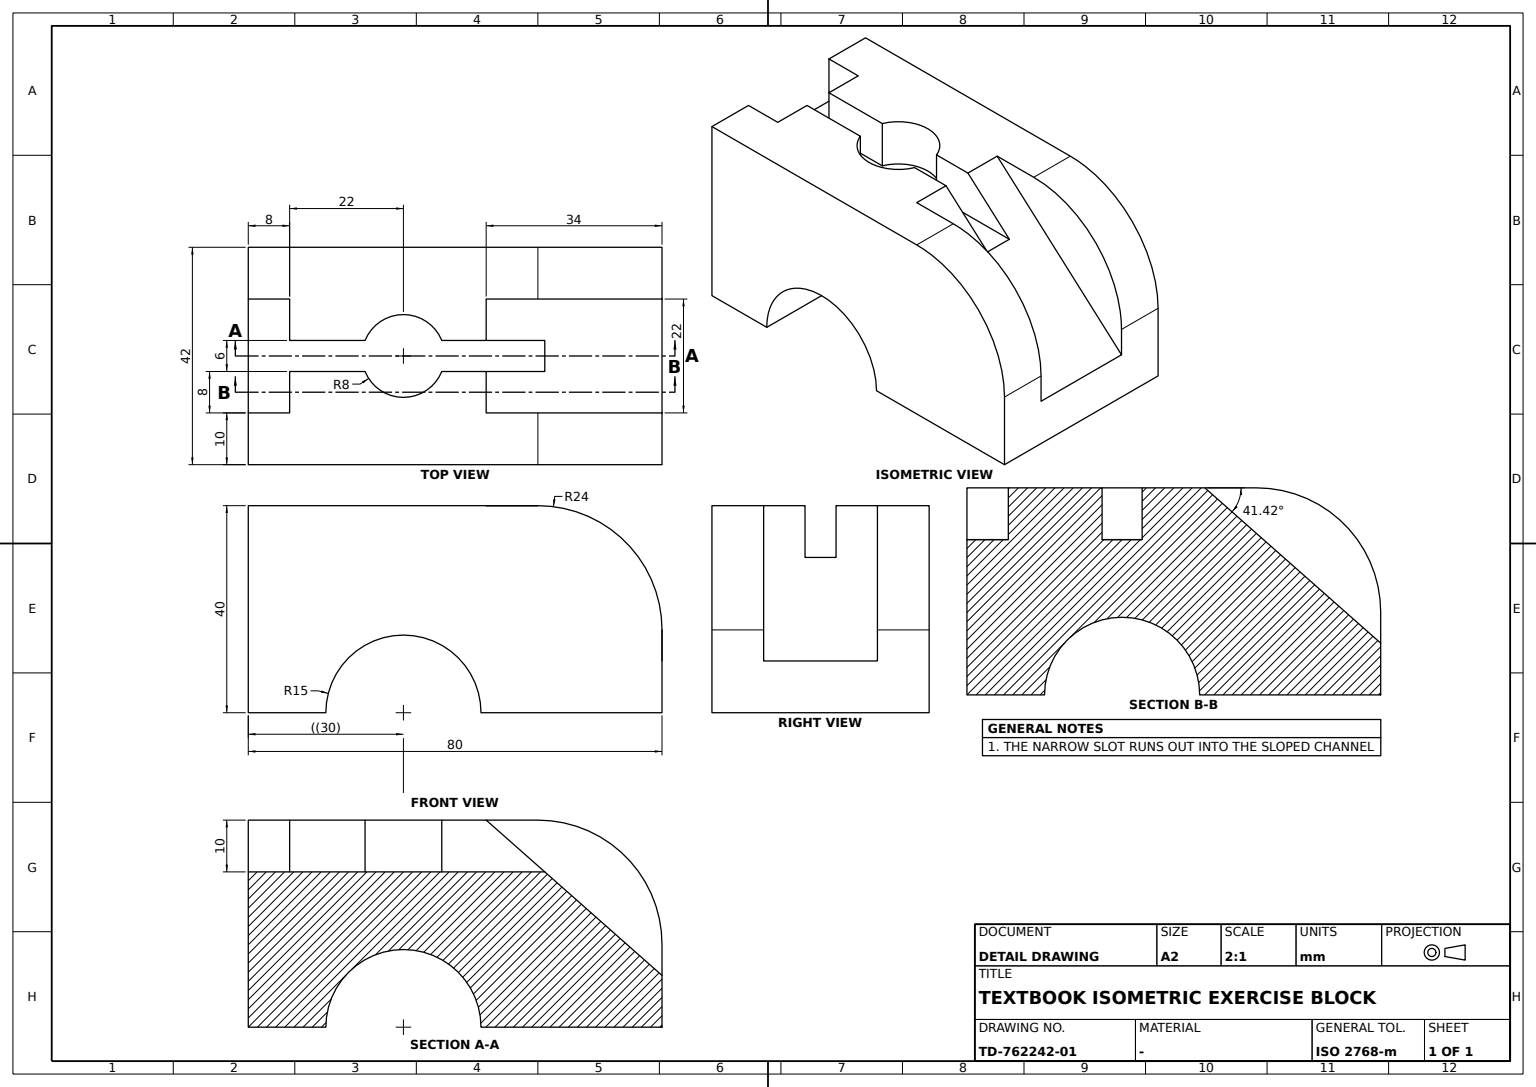
CATIA V5 part; units mm, degrees
sketch "Sketch1" plane through (0, 0, 0) normal (1, 0, 0) x (0, 1, 0)
  line L0 (0, 0) -> (80, 0)
  line L1 (80, 0) -> (80, 40)
  line L2 (80, 40) -> (0, 40)
  line L3 (0, 40) -> (0, 0)
  dimension "length L1" = 40
  dimension "length L0" = 80
  constraint horizontal L0 x-axis
  constraint horizontal L2 x-axis
  constraint vertical L1 y-axis
  constraint vertical L3 y-axis
extrude "Pad1" add sketch "Sketch1" along normal mid plane 42
sketch "Sketch2" plane through (21, 0, 0) normal (1, 0, 0) x (0, 1, 0)
  line L0 (80, 40) -> (46, 40)
  line L1 (46, 40) -> (80, 10)
  line L2 (80, 10) -> (80, 40)
  line L3 (80, 40) -> (0, 40) construction
  line L4 (80, 0) -> (80, 40) construction
  dimension "length L0" = 34
  dimension "length L2" = 30
  constraint horizontal L0 x-axis
  constraint vertical L2 y-axis
  constraint coincidence L0 L3
  constraint coincidence L4 L2
extrude "Pocket1" cut sketch "Sketch2" against normal up to next
sketch "Sketch3" plane through (21, 0, 0) normal (1, 0, 0) x (0, 1, 0)
  line L0 (46, 40) -> (80, 10)
  point P0 (80, 10)
  line L1 (80, 10) -> (80, 40)
  line L2 (80, 40) -> (46, 40)
  line L3 (46, 40) -> (80, 10) construction
  line L4 (80, 0) -> (80, 40) construction
  dimension "length L2" = 34
  constraint vertical L1 y-axis
  constraint horizontal L2 x-axis
  constraint coincidence L0 L3
  constraint coincidence P0 L4
extrude "Pad2" add sketch "Sketch3" against normal blind 10
sketch "Sketch4" plane through (-21, 0, 0) normal (-1, 0, 0) x (0, -1, 0)
  point P0 (-46, 40)
  line L0 (-46, 40) -> (-80, 10)
  line L1 (-80, 10) -> (-80, 40)
  line L2 (-80, 40) -> (-46, 40)
  line L3 (-46, 40) -> (-80, 10) construction
  point P1 (-46, 40)
  dimension "length L2" = 34
  constraint vertical L1 y-axis
  constraint coincidence L0 L3
  constraint coincidence P0 P1
  constraint horizontal L2 x-axis
extrude "Pad3" add sketch "Sketch4" against normal blind 10
fillet "Fillet1" radius 24 2 edges at (16, 80, 40) (-16, 80, 40)
sketch "Sketch5" plane through (0, 0, 40) normal (0, 0, 1) x (1, 0, 0)
  line L0 (-11, 8) -> (-3, 8)
  line L1 (11, 8) -> (11, 0)
  line L2 (11, 0) -> (-11, 0)
  line L3 (-11, 0) -> (-11, 8)
  line L4 (21, 80) -> (21, 0) construction
  line L5 (-21, 80) -> (-21, 0) construction
  arc A0 (3, 22.5838) -> (3, 37.4162) centre (0, 30) ccw
  point P0 (0, 30)
  line L6 (3, 22.5838) -> (3, 8)
  line L7 (-3, 8) -> (-3, 22.5838)
  line L8 (3, 8) -> (11, 8)
  line L9 (-3, 57.4162) -> (3, 57.4162)
  line L10 (3, 57.4162) -> (3, 37.4162)
  line L11 (-3, 37.4162) -> (-3, 57.4162)
  arc A1 (-3, 37.4162) -> (-3, 22.5838) centre (0, 30) ccw
  dimension "length L1" = 8
  dimension "distance L1 L4" = 10
  dimension "distance L3 L5" = 10
  dimension "radius A0" = 8
  dimension "distance P0 L0" = 22
  dimension "distance L6 L1" = 8
  dimension "length L10" = 20
  constraint horizontal L0 x-axis
  constraint horizontal L2 x-axis
  constraint horizontal L8 x-axis
  constraint horizontal L9 x-axis
  constraint vertical L1 y-axis
  constraint vertical L3 y-axis
  constraint vertical L6 y-axis
  constraint vertical L7 y-axis
  constraint vertical L10 y-axis
  constraint vertical L11 y-axis
  constraint coincidence x-axis L2
  constraint coincidence P0 y-axis
  constraint coincidence L0 L8
  constraint coincidence A0 A1
extrude "Pocket2" cut sketch "Sketch5" against normal blind 10
sketch "Sketch6" plane through (21, 0, 0) normal (1, 0, 0) x (0, 1, 0)
  circle A0 centre (30, 0) radius 15
  point P0 (30, 0)
  dimension "radius A0" = 15
  dimension "distance P0 y axis" = 30
  constraint coincidence P0 x-axis
extrude "Pocket3" cut sketch "Sketch6" against normal up to next
properties part number "catia 27"
